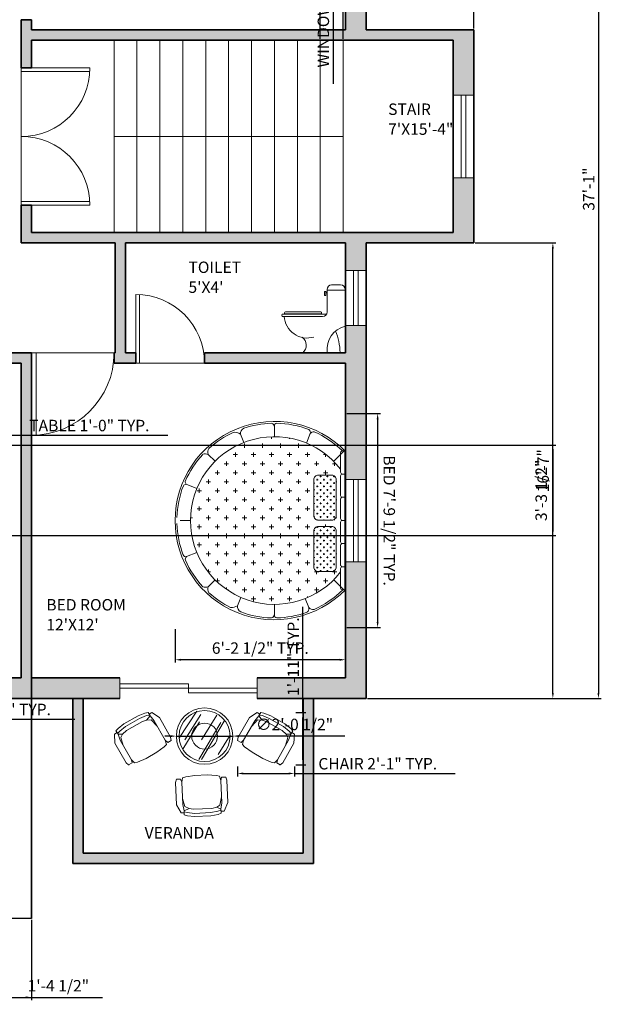
# Model space of a CAD drawing. Units: inches. Extents: x 2923 to 3500, y 1684 to 2381.
# Tile 9 of 12: x 3246 to 3500, y 1684 to 2114. Entities that reach past the tile are written whole.
import ezdxf

# ---------------------------------------------------------------- set-up
doc = ezdxf.new("R2010")
doc.units = ezdxf.units.IN
for name, color, linetype, lineweight in [('A-ANNO-DIMS', 2, 'Continuous', 18), ('A-AREA-IDEN', 7, 'Continuous', 18), ('A-DOOR', 3, 'Continuous', 18), ('A-FLOR-FIXT', 8, 'Continuous', 18), ('A-FLOR-OTLN', 7, 'Continuous', 25), ('A-FLOR-STRS', 7, 'Continuous', 18), ('A-FURN-PATT', 8, 'Continuous', 13), ('A-GLAZ', 4, 'Continuous', 18), ('A-WALL', 7, 'Continuous', 35), ('A-WALL-PATT', 9, 'Continuous', 13), ('Furniture', 7, 'Continuous', 15)]:
    doc.layers.add(name, color=color, linetype=linetype, lineweight=lineweight)
doc.styles.get("Standard").update_dxf_attribs({"font": 'txt', "height": 5})
doc.dimstyles.new('ISO-25', dxfattribs={"dimtxt": 5, "dimasz": 2.5, "dimexe": 1.25, "dimexo": 0.625, "dimtad": 1, "dimlunit": 3, "dimtxsty": 'Standard', "dimcen": 2.5, "dimadec": 0, "dimazin": 0, "dimtfac": 1, "dimtmove": 0, "dimatfit": 3, "dimfxl": 1, "dimarcsym": 0})

# ---------------------------------------------------------------- blocks, each defined once
blk = doc.blocks.new('*D3')
at = {"layer": 'A-ANNO-DIMS', "color": 0, "lineweight": -2, "transparency": 16777216}
for p, q in [((3397.85, 2262.41), (3499.87, 2262.41)), ((3498.62, 2259.91), (3498.62, 1819.91)), ((3397.85, 1817.41), (3499.87, 1817.41))]:
    blk.add_line(p, q, dxfattribs=at)
at = {"layer": 'A-ANNO-DIMS', "color": 0, "transparency": 16777216}
for points in [[(3498.2, 2259.91), (3499.04, 2259.91), (3498.62, 2262.41)], [(3498.2, 1819.91), (3499.04, 1819.91), (3498.62, 1817.41)]]:
    blk.add_solid(points, dxfattribs=at)
at = {"layer": 'Defpoints', "color": 0, "transparency": 16777216}
for p in [(3397.23, 2262.41), (3397.23, 1817.41), (3498.62, 1817.41)]:
    blk.add_point(p, dxfattribs=at)
at = {"layer": 'A-ANNO-DIMS', "color": 0, "transparency": 16777216, "insert": (3495.02, 2039.91), "char_height": 5, "attachment_point": 5, "rotation": 90}
blk.add_mtext('37\'-1"', dxfattribs=at)
blk = doc.blocks.new('DOOR-SINGLE-36IN')
for p, q in [((36, 36), (0, 36)), ((34, 0.06), (34, 36)), ((36, 0), (36, 36))]:
    blk.add_line(p, q)
blk.add_arc((36, 36), 36, 180, 270)
blk = doc.blocks.new('DOOR-SINGLE-30IN')
for p, q in [((0, 30), (0, 0)), ((1.67, 29.95), (1.67, 0)), ((0, 0), (30, 0))]:
    blk.add_line(p, q)
blk.add_arc((0, 0), 30, 0, 90)
blk = doc.blocks.new('DOOR-PAIR-60IN')
for p, q in [((0, 30), (0, 0)), ((1.67, 29.95), (1.67, 0)), ((58.33, 29.95), (58.33, 0)), ((60, 30), (60, 0)), ((0, 0), (30, 0)), ((60, 0), (30, 0))]:
    blk.add_line(p, q)
for centre, start, end in [((0, 0), 0, 90), ((60, 0), 90, 180)]:
    blk.add_arc(centre, 30, start, end)
blk = doc.blocks.new('WINDOW-36IN')
for p, q in [((36, 9), (0, 9)), ((0, 9), (0, 0)), ((36, 0), (36, 9)), ((36, 5.5), (0, 5.5)), ((36, 3.5), (0, 3.5)), ((0, 0), (36, 0))]:
    blk.add_line(p, q)
blk = doc.blocks.new('WINDOW-SLIDING-60IN')
for p, q in [((0, 0), (0, 9)), ((60, 0), (60, 9)), ((60, 4.5), (0, 4.5)), ((30, 4.5), (30, 6.5)), ((30, 6.5), (60, 6.5)), ((30, 4.5), (30, 2.5)), ((30, 2.5), (0, 2.5))]:
    blk.add_line(p, q)
blk = doc.blocks.new('VERANDA-PARAPET')
for p, q in [((0, 72), (0, 0)), ((4.5, 72), (4.5, 4.5)), ((100.5, 72), (100.5, 4.5)), ((105, 72), (105, 0)), ((100.5, 4.5), (4.5, 4.5)), ((105, 0), (0, 0))]:
    blk.add_line(p, q)
blk = doc.blocks.new('WC-FLOOR-MOUNT')
for p, q in [((0, 27.6), (0, 11.63)), ((7.97, 27.41), (0.2, 27.41)), ((6.05, 29.7), (2.11, 29.7)), ((8.49, 26.69), (7.97, 26.69)), ((7.97, 26.69), (7.97, 26.28)), ((7.97, 26.28), (8.49, 26.28)), ((8.02, 27.73), (8.02, 17.89)), ((8.02, 26.69), (8.02, 26.28)), ((8.49, 26.28), (8.49, 26.69)), ((9.1, 26.79), (8.59, 26.79)), ((8.59, 26.79), (8.59, 25.06)), ((9.1, 25.06), (9.1, 26.79)), ((8.59, 25.06), (9.1, 25.06)), ((10.4, 17.5), (10.4, 17.11)), ((26.23, 17.89), (10.79, 17.89)), ((26.62, 17.11), (26.62, 17.5)), ((27.42, 16.99), (8.24, 16.99)), ((27.42, 15.92), (9.99, 15.92)), ((10.4, 17.11), (26.62, 17.11)), ((15.89, 17.11), (15.89, 16.99)), ((23.77, 17.11), (23.77, 16.99)), ((27.82, 16.6), (27.82, 16.32)), ((18.71, 0.04), (2.25, 0.04)), ((8.02, 2.66), (8.02, 0.17)), ((8.02, 2.66), (8.02, 0.17))]:
    blk.add_line(p, q)
for centre, radius, start, end in [((2.11, 27.73), 1.97, 90, 180), ((6.05, 27.73), 1.97, 0, 90), ((9.99, 17.89), 1.97, 180, 270), ((10.79, 17.5), 0.394, 90, 180), ((26.23, 17.5), 0.394, 0, 90), ((16.71, 16.55), 10.05, 252.943, 356.7365), ((27.42, 16.6), 0.394, 0, 90), ((27.42, 16.32), 0.394, 270, 0), ((-2.41, 1.48), 10.5, 353.9182, 75.9043), ((31.43, -1.03), 29.12, 158.693, 177.6281), ((21.51, 3.3), 4.38, 125.5613, 228.8008)]:
    blk.add_arc(centre, radius, start, end)
blk = doc.blocks.new('BED-ROUND-FRAME')
for p, q in [((31.04, 79.92), (31.04, 84.58)), ((31.04, 79.92), (31.04, 84.58)), ((17.61, 77.37), (16.05, 81.29)), ((45.66, 76.84), (47.11, 80.49)), ((0, 13.11), (0, 73.51)), ((5.15, 69.2), (0.74, 73.61)), ((5.15, 69.2), (0.74, 73.61)), ((56.93, 69.2), (59.95, 72.21)), ((56.93, 69.2), (59.95, 72.21)), ((59.95, 72.21), (56.93, 69.2)), ((13.83, 63.84), (13.83, 47.62)), ((64.9, 57.24), (69.31, 59.05)), ((69.31, 59.05), (69.4, 59.09)), ((67.65, 43.31), (72.18, 43.31)), ((13.83, 41.4), (13.83, 25.18)), ((13.83, 39.13), (13.84, 39.12)), ((64.9, 29.37), (69.53, 27.47)), ((0.42, 12.68), (5.15, 17.42)), ((0.42, 12.68), (5.15, 17.42)), ((59.95, 14.4), (56.93, 17.42)), ((17.07, 9.46), (15.35, 5.25)), ((44.42, 9.23), (45.86, 5.58)), ((31.04, 1.98), (31.04, 6.69)), ((31.04, 2.04), (31.04, 6.69))]:
    blk.add_line(p, q)
for points in [[(4, 47.85), (4, 63.6, -0.414214), (5.97, 65.57), (11.88, 65.57, -0.414214), (13.84, 63.6), (13.84, 47.85, -0.414214), (11.88, 45.89), (5.97, 45.89, -0.414214)], [(4, 25.41), (4, 41.16, -0.414214), (5.97, 43.13), (11.88, 43.13, -0.414214), (13.84, 41.16), (13.84, 25.41, -0.414214), (11.88, 23.45), (5.97, 23.45, -0.414214)]]:
    blk.add_lwpolyline(points, format="xyb", close=True)
for centre, radius, start, end in [((31.04, 43.31), 43.31, 224.213, 135.787), ((31.04, 43.31), 42.52, 114.0695, 134.5949), ((14.23, 79.9), 2.29, 37.3562, 103.3498), ((17.88, 81.76), 1.88, 111.9527, 202.5488), ((31.04, 43.31), 42.52, 91.3819, 109.0292), ((29.76, 84.56), 1.29, 359.0498, 78.348), ((32.5, 84.36), 1.46, 98.688, 183.9778), ((31.04, 43.31), 42.52, 69.8397, 88.3303), ((44.67, 80.98), 2.46, 345.7709, 65.4979), ((31.04, 43.31), 36.61, 217.8198, 142.1802), ((49.64, 77.03), 4.29, 82.908, 126.1659), ((31.04, 43.31), 42.52, 47.802, 63.2705), ((57.53, 73.21), 2.61, 337.5919, 37.6583), ((61.1, 69.09), 3.33, 70.4217, 110.1689), ((31.04, 43.31), 42.52, 24.0703, 42.854), ((68.6, 60.18), 1.35, 304.4266, 20.4145), ((69.6, 57.73), 1.36, 26.1665, 102.6069), ((31.04, 43.31), 42.52, 1.7281, 20.7271), ((31.04, 43.31), 42.52, 339.0428, 358.2719), ((31.04, 43.31), 42.52, 317.146, 336.245), ((69.4, 29.21), 1.75, 274.2316, 320.4352), ((68.35, 26.36), 1.62, 353.6066, 43.1756), ((57.53, 13.4), 2.61, 322.3417, 22.4081), ((61.1, 17.52), 3.33, 249.8311, 289.5783), ((31.04, 43.31), 42.52, 225.7269, 245.8957), ((31.04, 43.31), 42.52, 295.113, 312.198), ((13.85, 6.32), 1.83, 264.4179, 326.0029), ((16.89, 4.85), 1.59, 153.9459, 235.5493), ((42.79, 5.51), 3.04, 302.4304, 3.4261), ((48.39, 9.04), 4.29, 233.8341, 279.2916), ((31.04, 43.31), 42.52, 249.2703, 268.6181), ((29.76, 2.06), 1.29, 281.652, 0.9502), ((32.5, 2.25), 1.46, 176.0222, 261.312), ((31.04, 43.31), 42.52, 271.6697, 288.3347)]:
    blk.add_arc(centre, radius, start, end)
blk = doc.blocks.new('CHAIR-VERANDA')
for p, q in [((5.19, 20.65), (8.53, 22.86)), ((8.53, 22.86), (9.7, 22.19)), ((9.25, 21.41), (9.7, 22.19)), ((9.47, 21.8), (10.86, 21.52)), ((9.7, 22.19), (10.14, 22.96)), ((10.14, 22.96), (11.53, 22.68)), ((10.86, 21.52), (13.8, 20.34)), ((11.53, 22.68), (14.47, 21.51)), ((14.47, 21.51), (20.68, 17.94)), ((0.28, 12.11), (5.19, 20.65)), ((7.52, 19.31), (2.61, 10.77)), ((6.18, 16.98), (8.75, 19.64)), ((9.25, 21.41), (7.52, 19.31)), ((8.75, 19.64), (10.75, 19.52)), ((10.75, 19.52), (9.25, 21.41)), ((12.52, 19.01), (10.75, 19.52)), ((19.51, 14.99), (12.52, 19.01)), ((13.8, 20.34), (20.01, 16.77)), ((20.68, 17.94), (23.18, 15.98)), ((21.23, 13.49), (19.51, 14.99)), ((20.01, 16.77), (22.51, 14.82)), ((23.23, 13.37), (21.23, 13.49)), ((21.94, 12.04), (21.23, 13.49)), ((23.23, 13.37), (22.27, 10.82)), ((22.51, 14.82), (23.45, 13.76)), ((23.18, 15.98), (24.12, 14.93)), ((23.67, 14.15), (23.23, 13.37)), ((24.12, 14.93), (23.67, 14.15)), ((23.67, 14.15), (24.84, 13.48)), ((24.84, 13.48), (24.6, 9.48)), ((0, 10.72), (0.28, 12.11)), ((1.55, 9.82), (0, 10.72)), ((2.61, 10.77), (1.55, 9.82)), ((2.11, 8.99), (2.61, 10.77)), ((3.05, 7.93), (2.11, 8.99)), ((22.27, 10.82), (17.36, 2.28)), ((24.6, 9.48), (19.69, 0.94)), ((20.93, 8.49), (21.94, 12.04)), ((21.26, 9.64), (21.6, 9.64)), ((6.32, 5.53), (3.05, 7.93)), ((10.98, 2.85), (6.32, 5.53)), ((14.69, 1.23), (10.98, 2.85)), ((16.08, 0.95), (14.69, 1.23)), ((17.36, 2.28), (16.08, 0.95)), ((17.08, 0.89), (17.36, 2.28)), ((18.63, 0), (17.08, 0.89)), ((18.36, 0.02), (18.6, 0.02)), ((19.69, 0.94), (18.63, 0))]:
    blk.add_line(p, q)
blk = doc.blocks.new('*D19')
at = {"layer": 'A-ANNO-DIMS', "color": 0, "lineweight": -2, "transparency": 16777216}
for p, q in [((3387.6, 2199.41), (3381.58, 2199.41)), ((3382.83, 2196.91), (3382.83, 2165.91)), ((3387.6, 2163.41), (3381.58, 2163.41)), ((3382.83, 2163.41), (3382.83, 2085.85))]:
    blk.add_line(p, q, dxfattribs=at)
at = {"layer": 'A-ANNO-DIMS', "color": 0, "transparency": 16777216}
for points in [[(3382.41, 2196.91), (3383.25, 2196.91), (3382.83, 2199.41)], [(3382.41, 2165.91), (3383.25, 2165.91), (3382.83, 2163.41)]]:
    blk.add_solid(points, dxfattribs=at)
at = {"layer": 'Defpoints', "color": 0, "transparency": 16777216}
for p in [(3388.23, 2199.41), (3382.83, 2163.41), (3388.23, 2163.41)]:
    blk.add_point(p, dxfattribs=at)
at = {"layer": 'A-ANNO-DIMS', "color": 0, "transparency": 16777216, "insert": (3379.23, 2123.38), "char_height": 5, "attachment_point": 5, "rotation": 90}
blk.add_mtext('WINDOW 3\'-0" TYP.', dxfattribs=at)
blk = doc.blocks.new('*D29')
at = {"layer": 'A-ANNO-DIMS', "color": 0, "lineweight": -2, "transparency": 16777216}
for p, q in [((3119.23, 1816.78), (3119.23, 1807.16)), ((3179.23, 1816.78), (3179.23, 1807.16)), ((3121.73, 1808.41), (3176.73, 1808.41)), ((3179.23, 1808.41), (3270.12, 1808.41))]:
    blk.add_line(p, q, dxfattribs=at)
at = {"layer": 'A-ANNO-DIMS', "color": 0, "transparency": 16777216}
for points in [[(3121.73, 1808.82), (3121.73, 1807.99), (3119.23, 1808.41)], [(3176.73, 1808.82), (3176.73, 1807.99), (3179.23, 1808.41)]]:
    blk.add_solid(points, dxfattribs=at)
at = {"layer": 'Defpoints', "color": 0, "transparency": 16777216}
for p in [(3119.23, 1817.41), (3179.23, 1817.41), (3179.23, 1808.41)]:
    blk.add_point(p, dxfattribs=at)
at = {"layer": 'A-ANNO-DIMS', "color": 0, "transparency": 16777216, "insert": (3225.93, 1812.01), "char_height": 5, "attachment_point": 5}
blk.add_mtext('DOOR PAIR 5\'-0" TYP.', dxfattribs=at)
blk = doc.blocks.new('*D33')
at = {"layer": 'A-ANNO-DIMS', "color": 0, "lineweight": -2, "transparency": 16777216}
for p, q in [((3388.85, 1941.91), (3403.51, 1941.91)), ((3402.26, 1939.41), (3402.26, 1850.9)), ((3388.86, 1848.4), (3403.51, 1848.4))]:
    blk.add_line(p, q, dxfattribs=at)
at = {"layer": 'A-ANNO-DIMS', "color": 0, "transparency": 16777216}
for points in [[(3402.67, 1939.41), (3401.84, 1939.41), (3402.26, 1941.91)], [(3402.67, 1850.9), (3401.84, 1850.9), (3402.26, 1848.4)]]:
    blk.add_solid(points, dxfattribs=at)
at = {"layer": 'Defpoints', "color": 0, "transparency": 16777216}
for p in [(3388.23, 1941.91), (3388.23, 1848.4), (3402.26, 1848.4)]:
    blk.add_point(p, dxfattribs=at)
at = {"layer": 'A-ANNO-DIMS', "color": 0, "transparency": 16777216, "insert": (3406.69, 1895.16), "char_height": 5, "attachment_point": 5, "rotation": 270.0003}
blk.add_mtext('BED 7\'-9 1/2" TYP.', dxfattribs=at)
blk = doc.blocks.new('*D34')
at = {"layer": 'A-ANNO-DIMS', "color": 0, "lineweight": -2, "transparency": 16777216}
for p, q in [((3313.88, 1847.78), (3313.88, 1833.12)), ((3388.23, 1847.78), (3388.23, 1833.12)), ((3385.73, 1834.37), (3316.38, 1834.37))]:
    blk.add_line(p, q, dxfattribs=at)
at = {"layer": 'A-ANNO-DIMS', "color": 0, "transparency": 16777216}
for points in [[(3316.38, 1834.79), (3316.38, 1833.96), (3313.88, 1834.37)], [(3385.73, 1834.79), (3385.73, 1833.96), (3388.23, 1834.37)]]:
    blk.add_solid(points, dxfattribs=at)
at = {"layer": 'Defpoints', "color": 0, "transparency": 16777216}
for p in [(3313.88, 1848.4), (3388.23, 1848.4), (3313.88, 1834.37)]:
    blk.add_point(p, dxfattribs=at)
at = {"layer": 'A-ANNO-DIMS', "color": 0, "transparency": 16777216, "insert": (3351.06, 1838.81), "char_height": 5, "attachment_point": 5, "rotation": 0.0003}
blk.add_mtext('6\'-2 1/2" TYP.', dxfattribs=at)
blk = doc.blocks.new('*D45')
at = {"layer": 'A-ANNO-DIMS', "color": 0, "lineweight": -2, "transparency": 16777216}
for p, q in [((3227.9, 1933.56), (3227.9, 1931.16)), ((3230.4, 1932.41), (3237.25, 1932.41)), ((3239.75, 1933.56), (3239.75, 1931.16)), ((3239.75, 1932.41), (3310.64, 1932.41))]:
    blk.add_line(p, q, dxfattribs=at)
at = {"layer": 'A-ANNO-DIMS', "color": 0, "transparency": 16777216}
for points in [[(3230.4, 1932.83), (3230.4, 1931.99), (3227.9, 1932.41)], [(3237.25, 1932.83), (3237.25, 1931.99), (3239.75, 1932.41)]]:
    blk.add_solid(points, dxfattribs=at)
at = {"layer": 'Defpoints', "color": 0, "transparency": 16777216}
for p in [(3227.9, 1934.19), (3239.75, 1934.19), (3239.75, 1932.41)]:
    blk.add_point(p, dxfattribs=at)
at = {"layer": 'A-ANNO-DIMS', "color": 0, "transparency": 16777216, "insert": (3276.45, 1936.01), "char_height": 5, "attachment_point": 5}
blk.add_mtext('TABLE 1\'-0" TYP.', dxfattribs=at)
blk = doc.blocks.new('*D47')
at = {"layer": 'A-ANNO-DIMS', "color": 0, "lineweight": -2, "transparency": 16777216}
for p, q in [((3341.13, 1787.8), (3341.13, 1783.45)), ((3343.63, 1784.7), (3363.47, 1784.7)), ((3365.97, 1787.8), (3365.97, 1783.45)), ((3365.97, 1784.7), (3436.15, 1784.7))]:
    blk.add_line(p, q, dxfattribs=at)
at = {"layer": 'A-ANNO-DIMS', "color": 0, "transparency": 16777216}
for points in [[(3343.63, 1785.12), (3343.63, 1784.29), (3341.13, 1784.7)], [(3363.47, 1785.12), (3363.47, 1784.29), (3365.97, 1784.7)]]:
    blk.add_solid(points, dxfattribs=at)
at = {"layer": 'Defpoints', "color": 0, "transparency": 16777216}
for p in [(3341.13, 1788.43), (3365.97, 1788.43), (3365.97, 1784.7)]:
    blk.add_point(p, dxfattribs=at)
at = {"layer": 'A-ANNO-DIMS', "color": 0, "transparency": 16777216, "insert": (3402.31, 1788.3), "char_height": 5, "attachment_point": 5}
blk.add_mtext('CHAIR 2\'-1" TYP.', dxfattribs=at)
blk = doc.blocks.new('*D48')
at = {"layer": 'A-ANNO-DIMS', "color": 0, "lineweight": -2, "transparency": 16777216}
for p, q in [((3369.69, 1811.39), (3369.69, 1857.52)), ((3366.59, 1811.39), (3370.94, 1811.39)), ((3369.69, 1790.93), (3369.69, 1808.89)), ((3366.59, 1788.43), (3370.94, 1788.43))]:
    blk.add_line(p, q, dxfattribs=at)
at = {"layer": 'A-ANNO-DIMS', "color": 0, "transparency": 16777216}
for points in [[(3369.28, 1808.89), (3370.11, 1808.89), (3369.69, 1811.39)], [(3369.28, 1790.93), (3370.11, 1790.93), (3369.69, 1788.43)]]:
    blk.add_solid(points, dxfattribs=at)
at = {"layer": 'Defpoints', "color": 0, "transparency": 16777216}
for p in [(3365.97, 1811.39), (3369.69, 1811.39), (3365.97, 1788.43)]:
    blk.add_point(p, dxfattribs=at)
at = {"layer": 'A-ANNO-DIMS', "color": 0, "transparency": 16777216, "insert": (3366.09, 1835.71), "char_height": 5, "attachment_point": 5, "rotation": 90}
blk.add_mtext('1\'-11" TYP.', dxfattribs=at)
blk = doc.blocks.new('*D49')
at = {"layer": 'A-ANNO-DIMS', "color": 0, "lineweight": -2, "transparency": 16777216}
for p, q in [((2969.23, 2263.03), (2969.23, 2370.16)), ((3444.23, 2110.03), (3444.23, 2370.16)), ((2971.73, 2368.91), (3441.73, 2368.91))]:
    blk.add_line(p, q, dxfattribs=at)
at = {"layer": 'A-ANNO-DIMS', "color": 0, "transparency": 16777216}
for points in [[(2971.73, 2369.32), (2971.73, 2368.49), (2969.23, 2368.91)], [(3441.73, 2369.32), (3441.73, 2368.49), (3444.23, 2368.91)]]:
    blk.add_solid(points, dxfattribs=at)
at = {"layer": 'Defpoints', "color": 0, "transparency": 16777216}
for p in [(3444.23, 2368.91), (2969.23, 2262.41), (3444.23, 2109.41)]:
    blk.add_point(p, dxfattribs=at)
at = {"layer": 'A-ANNO-DIMS', "color": 0, "transparency": 16777216, "insert": (3206.73, 2372.51), "char_height": 5, "attachment_point": 5}
blk.add_mtext('39\'-7"', dxfattribs=at)
blk = doc.blocks.new('*D59')
at = {"layer": 'A-ANNO-DIMS', "color": 0, "lineweight": -2, "transparency": 16777216}
for p, q in [((3444.85, 2016.41), (3479.98, 2016.41)), ((3478.73, 1819.91), (3478.73, 2013.91)), ((3397.85, 1817.41), (3479.98, 1817.41))]:
    blk.add_line(p, q, dxfattribs=at)
at = {"layer": 'A-ANNO-DIMS', "color": 0, "transparency": 16777216}
for points in [[(3478.31, 2013.91), (3479.15, 2013.91), (3478.73, 2016.41)], [(3478.31, 1819.91), (3479.15, 1819.91), (3478.73, 1817.41)]]:
    blk.add_solid(points, dxfattribs=at)
at = {"layer": 'Defpoints', "color": 0, "transparency": 16777216}
for p in [(3444.23, 2016.41), (3478.73, 2016.41), (3397.23, 1817.41)]:
    blk.add_point(p, dxfattribs=at)
at = {"layer": 'A-ANNO-DIMS', "color": 0, "transparency": 16777216, "insert": (3475.13, 1916.91), "char_height": 5, "attachment_point": 5, "rotation": 90}
blk.add_mtext('16\'-7"', dxfattribs=at)
blk = doc.blocks.new('*D60')
at = {"layer": 'A-ANNO-DIMS', "color": 0, "lineweight": -2, "transparency": 16777216}
for p, q in [((3241.34, 1928.12), (3479.98, 1928.12)), ((3478.73, 1925.62), (3478.73, 1891.08)), ((3241.34, 1888.58), (3479.98, 1888.58))]:
    blk.add_line(p, q, dxfattribs=at)
at = {"layer": 'A-ANNO-DIMS', "color": 0, "transparency": 16777216}
for points in [[(3478.31, 1925.62), (3479.15, 1925.62), (3478.73, 1928.12)], [(3478.31, 1891.08), (3479.15, 1891.08), (3478.73, 1888.58)]]:
    blk.add_solid(points, dxfattribs=at)
at = {"layer": 'Defpoints', "color": 0, "transparency": 16777216}
for p in [(3240.72, 1928.12), (3240.72, 1888.58), (3478.73, 1888.58)]:
    blk.add_point(p, dxfattribs=at)
at = {"layer": 'A-ANNO-DIMS', "color": 0, "transparency": 16777216, "insert": (3474.3, 1908.35), "char_height": 5, "attachment_point": 5, "rotation": 90}
blk.add_mtext('3\'-3 1/2"', dxfattribs=at)
blk = doc.blocks.new('*D61')
at = {"layer": 'A-ANNO-DIMS', "color": 0, "lineweight": -2, "transparency": 16777216}
for p, q in [((3224.5, 1890.49), (3224.5, 1685.66)), ((3241.23, 1890.49), (3241.23, 1685.66)), ((3227, 1686.91), (3238.73, 1686.91)), ((3241.23, 1686.91), (3282.12, 1686.91))]:
    blk.add_line(p, q, dxfattribs=at)
at = {"layer": 'A-ANNO-DIMS', "color": 0, "transparency": 16777216}
for points in [[(3227, 1687.32), (3227, 1686.49), (3224.5, 1686.91)], [(3238.73, 1687.32), (3238.73, 1686.49), (3241.23, 1686.91)]]:
    blk.add_solid(points, dxfattribs=at)
at = {"layer": 'Defpoints', "color": 0, "transparency": 16777216}
for p in [(3224.5, 1891.12), (3241.23, 1891.12), (3241.23, 1686.91)]:
    blk.add_point(p, dxfattribs=at)
at = {"layer": 'A-ANNO-DIMS', "color": 0, "transparency": 16777216, "insert": (3262.92, 1691.34), "char_height": 5, "attachment_point": 5}
blk.add_mtext('1\'-4 1/2"', dxfattribs=at)
blk = doc.blocks.new('*D69')
at = {"layer": 'A-ANNO-DIMS', "color": 0, "lineweight": -2, "transparency": 16777216}
for p, q in [((3110.23, 1720.78), (3110.23, 1685.66)), ((3251.23, 1720.78), (3251.23, 1685.66)), ((3112.73, 1686.91), (3248.73, 1686.91))]:
    blk.add_line(p, q, dxfattribs=at)
at = {"layer": 'A-ANNO-DIMS', "color": 0, "transparency": 16777216}
for points in [[(3112.73, 1687.32), (3112.73, 1686.49), (3110.23, 1686.91)], [(3248.73, 1687.32), (3248.73, 1686.49), (3251.23, 1686.91)]]:
    blk.add_solid(points, dxfattribs=at)
at = {"layer": 'Defpoints', "color": 0, "transparency": 16777216}
for p in [(3110.23, 1721.41), (3251.23, 1721.41), (3251.23, 1686.91)]:
    blk.add_point(p, dxfattribs=at)
at = {"layer": 'A-ANNO-DIMS', "color": 0, "transparency": 16777216, "insert": (3180.73, 1690.51), "char_height": 5, "attachment_point": 5}
blk.add_mtext('11\'-9"', dxfattribs=at)
blk = doc.blocks.new('*D71')
at = {"layer": 'A-ANNO-DIMS', "color": 0, "lineweight": -2, "transparency": 16777216}
for p, q in [((3377.23, 2105.53), (3377.23, 2370.16)), ((3387.23, 2105.53), (3387.23, 2370.16)), ((3379.73, 2368.91), (3384.73, 2368.91)), ((3387.23, 2368.91), (3414.55, 2368.91))]:
    blk.add_line(p, q, dxfattribs=at)
at = {"layer": 'A-ANNO-DIMS', "color": 0, "transparency": 16777216}
for points in [[(3379.73, 2369.32), (3379.73, 2368.49), (3377.23, 2368.91)], [(3384.73, 2369.32), (3384.73, 2368.49), (3387.23, 2368.91)]]:
    blk.add_solid(points, dxfattribs=at)
at = {"layer": 'Defpoints', "color": 0, "transparency": 16777216}
for p in [(3387.23, 2368.91), (3377.23, 2104.91), (3387.23, 2104.91)]:
    blk.add_point(p, dxfattribs=at)
at = {"layer": 'A-ANNO-DIMS', "color": 0, "transparency": 16777216, "insert": (3402.14, 2372.51), "char_height": 5, "attachment_point": 5}
blk.add_mtext('0\'-10"', dxfattribs=at)
blk = doc.blocks.new('*D73')
at = {"layer": 'A-ANNO-DIMS', "color": 0, "lineweight": -2, "transparency": 16777216}
for p, q in [((3311.94, 1801.02), (3309.44, 1801.02)), ((3314.44, 1801.02), (3339.07, 1801.03)), ((3387.94, 1801.03), (3341.57, 1801.03))]:
    blk.add_line(p, q, dxfattribs=at)
at = {"layer": 'A-ANNO-DIMS', "color": 0, "transparency": 16777216}
for points in [[(3311.94, 1801.44), (3311.94, 1800.61), (3314.44, 1801.02)], [(3341.57, 1801.44), (3341.57, 1800.61), (3339.07, 1801.03)]]:
    blk.add_solid(points, dxfattribs=at)
at = {"layer": 'Defpoints', "color": 0, "transparency": 16777216}
for p in [(3314.44, 1801.02), (3339.07, 1801.03)]:
    blk.add_point(p, dxfattribs=at)
at = {"layer": 'A-ANNO-DIMS', "color": 0, "transparency": 16777216, "insert": (3366, 1805.46), "char_height": 5, "attachment_point": 5, "rotation": 0.002}
blk.add_mtext('∅2\'-0 1/2"', dxfattribs=at)

msp = doc.modelspace()

# ---------------------------------------------------------------- hatches: boundary and pattern name
at = {"layer": 'A-FURN-PATT'}
h = msp.add_hatch(dxfattribs=at)
h.set_pattern_fill('CROSS', color=256, scale=15.748, angle=360, style=0)
h.set_pattern_definition([(180, (5120.696, 3404.2493), (-3.937, 3.937), [1.9685, -5.9055]), (90, (5119.7117, 3403.265), (3.937, 3.937), [1.9685, -5.9055])])
h.paths.add_polyline_path([(3386.112, 1872.705), (3386.112, 1874.251, -0.4142136), (3386.86, 1874.999, -0.4142136), (3386.112, 1875.747), (3386.112, 1884.371, -0.4142136), (3386.86, 1885.119, -0.4142136), (3386.112, 1885.867), (3386.112, 1894.492, -0.4142136), (3386.86, 1895.24, -0.4142136), (3386.112, 1895.988), (3386.112, 1904.612, -0.4142136), (3386.86, 1905.36, -0.4142136), (3386.112, 1906.108), (3386.112, 1914.733, -0.4142136), (3386.86, 1915.481, -0.4142136), (3386.112, 1916.229), (3386.112, 1917.607, 2.9191153)])
h.paths.add_polyline_path([(3374.386, 1913.05, -0.4142136), (3376.354, 1915.018), (3382.26, 1915.018, -0.4142136), (3384.228, 1913.05), (3384.228, 1897.302, -0.4142136), (3382.26, 1895.333), (3376.354, 1895.333, -0.4142136), (3374.386, 1897.302)], flags=16)
h.paths.add_polyline_path([(3376.354, 1892.577), (3382.26, 1892.577, -0.4142136), (3384.228, 1890.609), (3384.228, 1874.861, -0.4142136), (3382.26, 1872.892), (3376.354, 1872.892, -0.4142136), (3374.386, 1874.861), (3374.386, 1890.609, -0.4142136)], flags=16)
h = msp.add_hatch(dxfattribs=at)
h.set_pattern_fill('CROSS', color=256, scale=5.9055, angle=630, style=0)
h.set_pattern_definition([(270, (2643.6119, 2571.8263), (1.476375, -1.476375), [0.7381875, -2.2145625]), (360, (2643.2428, 2571.4572), (1.476375, 1.476375), [0.7381875, -2.2145625])])
h.paths.add_polyline_path([(3384.228, 1913.05, 0.4142136), (3382.26, 1915.018), (3376.354, 1915.018, 0.4142136), (3374.386, 1913.05), (3374.386, 1897.302, 0.4142136), (3376.354, 1895.333), (3382.26, 1895.333, 0.4142136), (3384.228, 1897.302)])
h.paths.add_polyline_path([(3374.386, 1874.861, 0.4142136), (3376.354, 1872.892), (3382.26, 1872.892, 0.4142136), (3384.228, 1874.861), (3384.228, 1890.609, 0.4142136), (3382.26, 1892.577), (3376.354, 1892.577, 0.4142136), (3374.386, 1890.609)])
at = {"layer": 'A-WALL-PATT'}
h = msp.add_hatch(color=256, dxfattribs=at)
h.dxf.hatch_style = 1
h.paths.add_polyline_path([(3014.23, 2262.406), (2969.23, 2262.406), (2969.23, 2201.5), (2978.23, 2201.5), (2978.23, 2213.699), (2978.23, 2253.406), (3014.23, 2253.406)])
h.paths.add_polyline_path([(3119.23, 2262.406), (3074.23, 2262.406), (3074.23, 2253.406), (3110.23, 2253.406), (3110.23, 2109.406), (3105.73, 2109.406), (3105.73, 2104.906), (3114.73, 2104.906), (3114.73, 2152.906), (3119.23, 2152.906), (3119.23, 2157.406), (3114.73, 2157.406), (3114.73, 2253.406), (3119.23, 2253.406)])
h.paths.add_polyline_path([(3179.98, 2262.406), (3149.23, 2262.406), (3149.23, 2253.406), (3179.98, 2253.406)], flags=0)
h.paths.add_polyline_path([(3295.73, 2262.406), (3215.98, 2262.406), (3215.98, 2253.406), (3246.73, 2253.406), (3246.73, 2157.406), (3149.23, 2157.406), (3149.23, 2152.906), (3246.73, 2152.906), (3246.73, 2149.906), (3251.23, 2149.906), (3251.23, 2253.406), (3295.73, 2253.406)])
h.paths.add_polyline_path([(3397.23, 2262.406), (3343.73, 2262.406), (3343.73, 2253.406), (3349.929, 2253.406), (3388.23, 2253.406), (3388.23, 2199.406), (3397.23, 2199.406)])
h.paths.add_polyline_path([(3369.935, 2334.406), (3264.935, 2334.406), (3264.935, 2262.406), (3269.435, 2262.406), (3269.435, 2329.906), (3365.435, 2329.906), (3365.435, 2262.406), (3369.935, 2262.406)])
h.paths.add_polyline_path([(3096.73, 2334.406), (2991.73, 2334.406), (2991.73, 2262.406), (2996.23, 2262.406), (2996.23, 2329.906), (3092.23, 2329.906), (3092.23, 2262.406), (3096.73, 2262.406)])
h.paths.add_polyline_path([(3397.23, 2163.406), (3388.23, 2163.406), (3388.23, 2109.406), (3251.23, 2109.406), (3251.23, 2113.906), (3246.73, 2113.906), (3246.73, 2092.906), (3251.23, 2092.906), (3251.23, 2104.906), (3435.23, 2104.906), (3435.23, 2080.906), (3444.23, 2080.906), (3444.23, 2109.406), (3397.23, 2109.406)])
h.paths.add_polyline_path([(3444.23, 2044.906), (3435.23, 2044.906), (3435.23, 2020.906), (3251.23, 2020.906), (3251.23, 2032.906), (3246.73, 2032.906), (3246.73, 2016.406), (3251.23, 2016.406), (3287.73, 2016.406), (3287.73, 1968.406), (3287.23, 1968.406), (3287.23, 1963.906), (3296.73, 1963.906), (3296.73, 1968.406), (3292.23, 1968.406), (3292.23, 2016.406), (3388.23, 2016.406), (3388.23, 2004.398), (3397.23, 2004.398), (3397.23, 2016.406), (3444.23, 2016.406)])
h.paths.add_polyline_path([(3397.23, 1980.398), (3388.23, 1980.398), (3388.23, 1979.998), (3388.23, 1969.828), (3388.23, 1968.406), (3326.73, 1968.406), (3326.73, 1963.906), (3388.23, 1963.906), (3388.23, 1913.156), (3397.23, 1913.156)])
h.paths.add_polyline_path([(3251.23, 1968.406), (3150.73, 1968.406), (3150.73, 1963.906), (3246.73, 1963.906), (3246.73, 1826.406), (3230.98, 1826.406), (3230.98, 1817.406), (3251.23, 1817.406), (3251.23, 1963.906)])
h.paths.add_polyline_path([(3114.73, 1968.406), (3105.73, 1968.406), (3105.73, 1963.906), (3110.23, 1963.906), (3110.23, 1817.406), (3119.23, 1817.406), (3119.23, 1826.406), (3114.73, 1826.406)])
h.paths.add_polyline_path([(3069.73, 1968.406), (3066.73, 1968.406), (3066.73, 1972.906), (3062.23, 1972.906), (3062.23, 1968.406), (2978.23, 1968.406), (2978.23, 1989.406), (2969.23, 1989.406), (2969.23, 1912.505), (2978.23, 1912.505), (2978.23, 1925.355), (2978.23, 1963.906), (3069.73, 1963.906)])
h.paths.add_polyline_path([(3066.73, 2104.906), (3069.73, 2104.906), (3069.73, 2109.406), (3057.73, 2109.406), (3057.73, 2104.906), (3062.23, 2104.906), (3062.23, 2038.906), (2978.23, 2038.906), (2978.23, 2059.906), (2969.23, 2059.906), (2969.23, 2013.406), (2978.23, 2013.406), (2978.23, 2034.406), (3062.23, 2034.406), (3062.23, 2002.906), (3066.73, 2002.906)])
h.paths.add_polyline_path([(3027.73, 2109.406), (2978.23, 2109.406), (2978.23, 2165.5), (2969.23, 2165.5), (2969.23, 2083.906), (2978.23, 2083.906), (2978.23, 2104.906), (3027.73, 2104.906)])
h.paths.add_polyline_path([(2978.23, 1876.505), (2969.23, 1876.505), (2969.23, 1817.406), (3014.23, 1817.406), (3014.23, 1826.406), (2978.23, 1826.406)])
h.paths.add_polyline_path([(2996.23, 1817.406), (2991.73, 1817.406), (2991.73, 1745.406), (3096.73, 1745.406), (3096.73, 1817.406), (3092.23, 1817.406), (3092.23, 1749.906), (2996.23, 1749.906)])
h.paths.add_polyline_path([(3289.73, 1826.406), (3251.23, 1826.406), (3251.23, 1817.406), (3289.73, 1817.406)])
h.paths.add_polyline_path([(3397.23, 1877.156), (3388.23, 1877.156), (3388.23, 1864.957), (3388.23, 1826.406), (3349.73, 1826.406), (3349.73, 1817.406), (3397.23, 1817.406)])
h.paths.add_polyline_path([(3374.267, 1817.406), (3369.767, 1817.406), (3369.767, 1749.906), (3273.767, 1749.906), (3273.767, 1817.406), (3269.267, 1817.406), (3269.267, 1745.406), (3374.267, 1745.406)])

# ---------------------------------------------------------------- linework, layer by layer
at = {"layer": 'A-FLOR-OTLN'}
msp.add_line((3251.23, 1721.406), (3110.23, 1721.406), dxfattribs=at)
at = {"layer": 'A-FLOR-STRS'}
for p, q in [((3287.23, 2020.906), (3287.23, 2104.906)), ((3297.23, 2020.906), (3297.23, 2104.906)), ((3307.23, 2020.906), (3307.23, 2104.906)), ((3317.23, 2020.906), (3317.23, 2104.906)), ((3327.23, 2020.906), (3327.23, 2104.906)), ((3337.23, 2020.906), (3337.23, 2104.906)), ((3347.23, 2020.906), (3347.23, 2104.906)), ((3357.23, 2020.906), (3357.23, 2104.906)), ((3367.23, 2020.906), (3367.23, 2104.906)), ((3377.23, 2020.906), (3377.23, 2104.906)), ((3387.23, 2020.906), (3387.23, 2104.906)), ((3287.23, 2062.906), (3387.23, 2062.906))]:
    msp.add_line(p, q, dxfattribs=at)
msp.add_lwpolyline([(3287.23, 2042.108, 0, 0, 0), (3401.78, 2042.108, 0, 0, 0), (3401.78, 2085.022, 0, 0, 0), (3293.654, 2085.022, 10, 0, 0), (3281.196, 2085.022, 0, 0, 0)], format="xyseb", dxfattribs=at)
at = {"layer": 'A-GLAZ'}
for p, q in [((3397.23, 2004.398), (3388.23, 2004.398)), ((3391.73, 1980.398), (3391.73, 2004.398)), ((3393.73, 1980.398), (3393.73, 2004.398)), ((3397.23, 1980.398), (3397.23, 2004.398)), ((3388.23, 1993.828), (3388.23, 1969.828)), ((3388.23, 1980.398), (3397.23, 1980.398)), ((3319.73, 1823.906), (3319.73, 1819.906)), ((3319.73, 1823.906), (3319.73, 1819.906))]:
    msp.add_line(p, q, dxfattribs=at)
at = {"layer": 'A-WALL'}
for p, q in [((3397.23, 2262.406), (3397.23, 2109.406)), ((3388.23, 2253.406), (3388.23, 2109.406)), ((3246.73, 2092.906), (3246.73, 2113.906)), ((3251.23, 2113.906), (3246.73, 2113.906)), ((3251.23, 2109.406), (3251.23, 2113.906)), ((3251.23, 2109.406), (3388.23, 2109.406)), ((3397.23, 2109.406), (3444.23, 2109.406)), ((3444.23, 2016.406), (3444.23, 2109.406)), ((3251.23, 2104.906), (3435.23, 2104.906)), ((3251.23, 2092.906), (3251.23, 2104.906)), ((3435.23, 2020.906), (3435.23, 2104.906)), ((3251.23, 2092.906), (3246.73, 2092.906)), ((3246.73, 2016.406), (3246.73, 2032.906)), ((3251.23, 2032.906), (3246.73, 2032.906)), ((3251.23, 2020.906), (3251.23, 2032.906)), ((3251.23, 2020.906), (3435.23, 2020.906)), ((3246.73, 2016.406), (3251.23, 2016.406)), ((3251.23, 2016.406), (3287.73, 2016.406)), ((3287.73, 2016.406), (3287.73, 1968.406)), ((3292.23, 2016.406), (3292.23, 1968.406)), ((3292.23, 2016.406), (3388.23, 2016.406)), ((3388.23, 2016.406), (3388.23, 1968.406)), ((3397.23, 2016.406), (3397.23, 1817.406)), ((3397.23, 2016.406), (3444.23, 2016.406)), ((3150.73, 1968.406), (3251.23, 1968.406)), ((3251.23, 1963.906), (3251.23, 1968.406)), ((3287.23, 1963.906), (3287.23, 1968.406)), ((3287.23, 1968.406), (3287.73, 1968.406)), ((3292.23, 1968.406), (3296.73, 1968.406)), ((3296.73, 1968.406), (3296.73, 1963.906)), ((3326.73, 1968.406), (3326.73, 1963.906)), ((3326.73, 1968.406), (3388.23, 1968.406)), ((3150.73, 1963.906), (3246.73, 1963.906)), ((3246.73, 1826.406), (3246.73, 1963.906)), ((3251.23, 1721.406), (3251.23, 1963.906)), ((3287.23, 1963.906), (3296.73, 1963.906)), ((3326.73, 1963.906), (3388.23, 1963.906)), ((3388.23, 1963.906), (3388.23, 1826.406)), ((3246.73, 1826.406), (3179.23, 1826.406)), ((3289.73, 1826.406), (3251.23, 1826.406)), ((3388.23, 1826.406), (3349.73, 1826.406)), ((3289.73, 1817.406), (3179.23, 1817.406)), ((3397.23, 1817.406), (3349.73, 1817.406))]:
    msp.add_line(p, q, dxfattribs=at)
at = {"layer": 'Furniture'}
for p, q in [((3315.487, 1799.923), (3323.363, 1811.894)), ((3318.113, 1799.339), (3325.113, 1810.434)), ((3320.99, 1810.553), (3320.99, 1810.319)), ((3317.238, 1795.252), (3324.53, 1807.222)), ((3324.238, 1790.872), (3333.864, 1806.93)), ((3325.405, 1799.339), (3332.114, 1810.142)), ((3325.405, 1790.872), (3335.322, 1807.514)), ((3332.697, 1792.916), (3337.947, 1801.383)), ((3314.503, 1782.187), (3314.114, 1780.826)), ((3314.114, 1780.826), (3314.542, 1770.983)), ((3316.292, 1782.265), (3314.503, 1782.187)), ((3316.798, 1780.942), (3316.292, 1782.265)), ((3317.168, 1782.751), (3316.798, 1780.942)), ((3317.226, 1771.099), (3316.798, 1780.942)), ((3318.491, 1783.257), (3317.168, 1782.751)), ((3322.498, 1783.88), (3318.491, 1783.257)), ((3327.867, 1784.113), (3322.498, 1783.88)), ((3331.913, 1783.841), (3327.867, 1784.113)), ((3333.275, 1783.452), (3331.913, 1783.841)), ((3333.8, 1781.682), (3333.275, 1783.452)), ((3334.189, 1783.043), (3333.8, 1781.682)), ((3334.228, 1771.838), (3333.8, 1781.682)), ((3335.978, 1783.121), (3334.189, 1783.043)), ((3336.484, 1781.798), (3335.978, 1783.121)), ((3336.912, 1771.955), (3336.484, 1781.798)), ((3317.109, 1773.784), (3318.16, 1770.243)), ((3334.111, 1774.523), (3333.372, 1770.905)), ((3333.897, 1769.135), (3334.228, 1771.838)), ((3335.278, 1768.298), (3336.912, 1771.955)), ((3314.542, 1770.983), (3316.487, 1767.481)), ((3316.487, 1767.481), (3317.829, 1767.539)), ((3317.79, 1768.434), (3317.226, 1771.099)), ((3319.988, 1769.426), (3317.79, 1768.434)), ((3317.79, 1768.434), (3317.829, 1767.539)), ((3317.81, 1767.987), (3319.171, 1767.598)), ((3317.829, 1767.539), (3317.868, 1766.645)), ((3318.16, 1770.243), (3319.988, 1769.426)), ((3319.171, 1767.598), (3322.323, 1767.287)), ((3321.797, 1769.057), (3319.988, 1769.426)), ((3329.851, 1769.407), (3321.797, 1769.057)), ((3322.323, 1767.287), (3329.481, 1767.598)), ((3329.481, 1767.598), (3332.594, 1768.181)), ((3332.068, 1769.952), (3329.851, 1769.407)), ((3333.372, 1770.905), (3332.068, 1769.952)), ((3333.897, 1769.135), (3332.068, 1769.952)), ((3332.594, 1768.181), (3333.916, 1768.687)), ((3333.936, 1768.24), (3333.897, 1769.135)), ((3333.936, 1768.24), (3335.278, 1768.298)), ((3333.975, 1767.345), (3333.936, 1768.24)), ((3317.868, 1766.645), (3319.23, 1766.256)), ((3319.23, 1766.256), (3322.381, 1765.944)), ((3322.381, 1765.944), (3329.54, 1766.256)), ((3329.54, 1766.256), (3332.652, 1766.839)), ((3332.652, 1766.839), (3333.975, 1767.345))]:
    msp.add_line(p, q, dxfattribs=at)
for points in [[(3386.112, 1924.853), (3386.112, 1916.229, 0.4142136), (3386.86, 1915.481), (3388.001, 1915.481), (3388.001, 1925.601), (3386.86, 1925.601, 0.4142136)], [(3386.112, 1914.733), (3386.112, 1906.108, 0.4142136), (3386.86, 1905.36), (3388.001, 1905.36), (3388.001, 1915.481), (3386.86, 1915.481, 0.4142136)], [(3386.112, 1904.612), (3386.112, 1895.988, 0.4142136), (3386.86, 1895.24), (3388.001, 1895.24), (3388.001, 1905.36), (3386.86, 1905.36, 0.4142136)], [(3386.112, 1894.492), (3386.112, 1885.867, 0.4142136), (3386.86, 1885.119), (3388.001, 1885.119), (3388.001, 1895.24), (3386.86, 1895.24, 0.4142136)], [(3386.112, 1884.371), (3386.112, 1875.747, 0.4142136), (3386.86, 1874.999), (3388.001, 1874.999), (3388.001, 1885.119), (3386.86, 1885.119, 0.4142136)], [(3386.112, 1874.251), (3386.112, 1865.627, 0.4142136), (3386.86, 1864.878), (3388.001, 1864.878), (3388.001, 1874.999), (3386.86, 1874.999, 0.4142136)]]:
    msp.add_lwpolyline(points, format="xyb", close=True, dxfattribs=at)
for radius in [12.316, 11.135, 5.645]:
    msp.add_circle((3326.752, 1801.025), radius, dxfattribs=at)

# ---------------------------------------------------------------- block references
at = {"layer": 'A-DOOR', "rotation": 270.0000000000021}
msp.add_blockref('DOOR-PAIR-60IN', (3246.73, 2092.906), dxfattribs=at)
at = {"layer": 'A-DOOR'}
msp.add_blockref('DOOR-SINGLE-30IN', (3296.73, 1963.906), dxfattribs=at)
at = {"layer": 'A-DOOR', "extrusion": (0, 0, -1), "zscale": -1}
msp.add_blockref('DOOR-SINGLE-36IN', (-3287.23, 1932.406), dxfattribs=at)
at = {"layer": 'A-FLOR-FIXT', "extrusion": (0, 0, -1), "zscale": -1}
msp.add_blockref('WC-FLOOR-MOUNT', (-3388.23, 1968.37), dxfattribs=at)
at = {"layer": 'A-GLAZ'}
for p, rotation in [((3435.23, 2080.906), 270.0000000000017), ((3388.23, 1913.156), 269.9999999999988)]:
    msp.add_blockref('WINDOW-36IN', p, dxfattribs=dict(at, rotation=rotation))
at = {"layer": 'A-GLAZ', "extrusion": (0, 0, -1), "zscale": -1}
msp.add_blockref('WINDOW-SLIDING-60IN', (-3349.73, 1817.406), dxfattribs=at)
at = {"layer": 'A-WALL'}
msp.add_blockref('VERANDA-PARAPET', (3269.267, 1745.406), dxfattribs=at)
at = {"layer": 'Furniture', "rotation": 180.0003415542786}
msp.add_blockref('BED-ROUND-FRAME', (3388.229, 1938.464), dxfattribs=at)
at = {"layer": 'Furniture', "extrusion": (0, 0, -1), "zscale": -1}
msp.add_blockref('CHAIR-VERANDA', (-3312.2, 1788.428), dxfattribs=at)
at = {"layer": 'Furniture'}
msp.add_blockref('CHAIR-VERANDA', (3341.131, 1788.428), dxfattribs=at)

# ---------------------------------------------------------------- texts
at = {"layer": 'A-AREA-IDEN'}
for s, p in [('STAIR', (3406.859, 2072.306)), ('7\'X15\'-4"', (3406.859, 2063.621)), ('TOILET', (3319.707, 2003.281)), ("5'X4'", (3319.707, 1994.596)), ('BED ROOM', (3257.679, 1855.877)), ("12'X12'", (3257.679, 1847.192)), ('VERANDA', (3300.586, 1756.293))]:
    msp.add_text(s, height=5, dxfattribs=at).set_placement(p)

# ---------------------------------------------------------------- dimensions: what is measured, and where the dimension line sits
at = {"layer": 'A-ANNO-DIMS'}
for base, p1, p2, picture, middle in [((3444.23, 2368.906), (2969.23, 2262.406), (3444.23, 2109.406), '*D49', (3206.73, 2372.507)), ((3387.23, 2368.906), (3377.23, 2104.906), (3387.23, 2104.906), '*D71', (3402.141, 2372.507)), ((3241.226, 1686.906), (3224.497, 1891.115), (3241.226, 1891.115), '*D61', (3262.923, 1691.341)), ((3251.23, 1686.906), (3110.23, 1721.406), (3251.23, 1721.406), '*D69', (3180.73, 1690.507))]:
    dim = msp.add_linear_dim(base=base, p1=p1, p2=p2, dimstyle='ISO-25', override={"dimdec": 1, "dimlfac": 1, "dimrnd": 0, "dimzin": 1, "dimdsep": 46, "dimlunit": 4, "dimfrac": 2}, dxfattribs=at)
    dim.commit()
    dim.dimension.update_dxf_attribs({"geometry": picture, "text_midpoint": middle})
for base, p1, p2, override, picture, middle in [((3498.62, 1817.406), (3397.23, 2262.406), (3397.23, 1817.406), {"dimclrd": 0, "dimclre": 0, "dimclrt": 0}, '*D3', (3495.019, 2039.906)), ((3478.73, 2016.406), (3397.23, 1817.406), (3444.23, 2016.406), {"dimdec": 1, "dimlfac": 1, "dimrnd": 0, "dimzin": 1, "dimdsep": 46, "dimlunit": 4, "dimfrac": 2}, '*D59', (3475.129, 1916.906)), ((3478.73, 1888.58), (3240.719, 1928.122), (3240.719, 1888.58), {"dimdec": 1, "dimlfac": 1, "dimrnd": 0, "dimzin": 1, "dimdsep": 46, "dimlunit": 4, "dimfrac": 2}, '*D60', (3474.295, 1908.351))]:
    dim = msp.add_linear_dim(base=base, p1=p1, p2=p2, angle=90, dimstyle='ISO-25', override=override, dxfattribs=at)
    dim.commit()
    dim.dimension.update_dxf_attribs({"geometry": picture, "text_midpoint": middle})
for base, p1, p2, angle, text, picture, middle in [((3382.83, 2163.406), (3388.23, 2199.406), (3388.23, 2163.406), 270, 'WINDOW <> TYP.', '*D19', (3379.229, 2123.376)), ((3402.257, 1848.401), (3388.23, 1941.913), (3388.23, 1848.401), 270.00034, 'BED <> TYP.', '*D33', (3406.691, 1895.157)), ((3369.694, 1811.393), (3365.968, 1788.428), (3365.968, 1811.393), 90, '<> TYP.', '*D48', (3366.093, 1835.708)), ((3313.883, 1834.374), (3388.23, 1848.401), (3313.883, 1848.4), 180.00034, '<> TYP.', '*D34', (3351.056, 1838.808))]:
    dim = msp.add_linear_dim(base=base, p1=p1, p2=p2, angle=angle, text=text, dimstyle='ISO-25', override={"dimdec": 1, "dimlfac": 1, "dimrnd": 0, "dimzin": 1, "dimdsep": 46, "dimlunit": 4, "dimfrac": 2}, dxfattribs=at)
    dim.commit()
    dim.dimension.update_dxf_attribs({"geometry": picture, "text_midpoint": middle})
for base, p1, p2, text, picture, middle in [((3239.7515, 1932.41), (3227.9018, 1934.1875), (3239.7515, 1934.1875), 'TABLE <> TYP.', '*D45', (3276.4479, 1936.0112)), ((3179.23, 1808.406), (3119.23, 1817.406), (3179.23, 1817.406), 'DOOR PAIR <> TYP.', '*D29', (3225.926, 1812.007)), ((3365.968, 1784.702), (3341.131, 1788.428), (3365.968, 1788.428), 'CHAIR <> TYP.', '*D47', (3402.308, 1788.303))]:
    dim = msp.add_linear_dim(base=base, p1=p1, p2=p2, text=text, dimstyle='ISO-25', override={"dimdec": 1, "dimlfac": 1, "dimrnd": 0, "dimzin": 1, "dimdsep": 46, "dimlunit": 4, "dimfrac": 2}, dxfattribs=at)
    dim.commit()
    dim.dimension.update_dxf_attribs({"geometry": picture, "text_midpoint": middle})
dim = msp.add_diameter_dim_2p(p1=(3314.436, 1801.024), p2=(3339.069, 1801.025), dimstyle='ISO-25', override={"dimdec": 1, "dimlfac": 1, "dimrnd": 0, "dimzin": 1, "dimdsep": 46, "dimlunit": 4, "dimfrac": 2}, dxfattribs=at)
dim.commit()
dim.dimension.update_dxf_attribs({"geometry": '*D73', "text_midpoint": (3366.003, 1801.026), "dimtype": 163})

doc.saveas('drawing.dxf')
